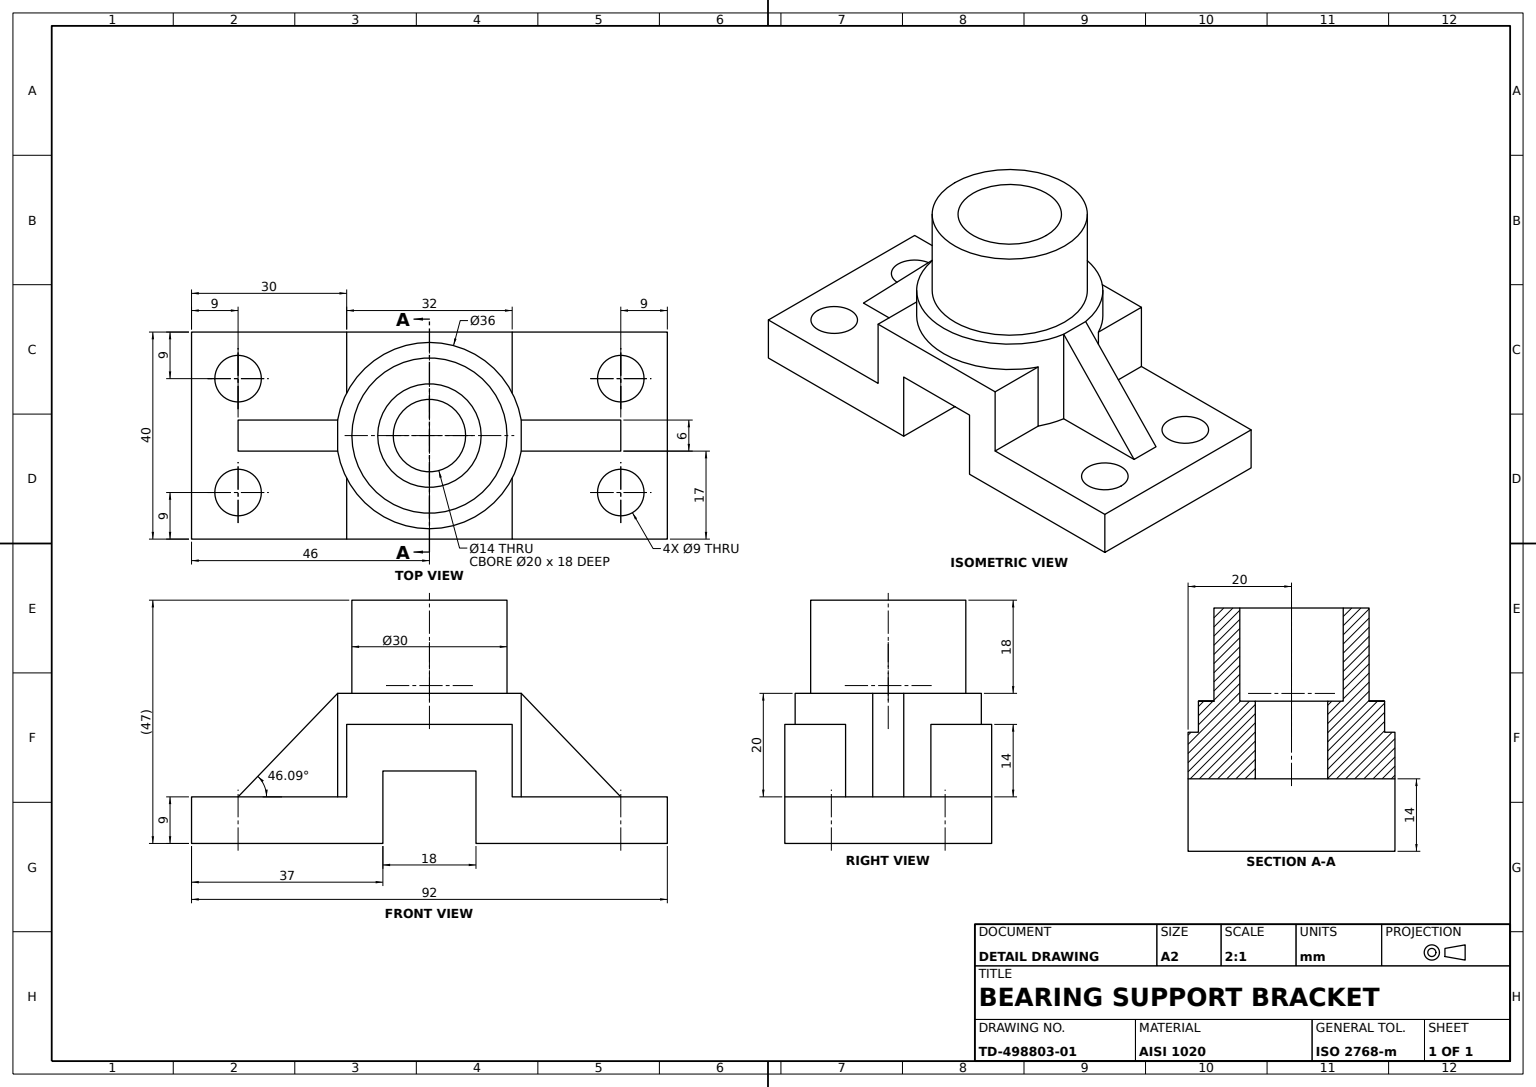
from build123d import *

# Parameters (mm, degrees)
STEPPED_BASE_DEPTH          = 20
COLLAR_36_SKETCH_R          = 18
COLLAR_36_DEPTH             = 20
COLLAR_TRIM_SKETCH_W        = 18
COLLAR_TRIM_SKETCH_H        = 5
COLLAR_TRIM_CUT_DEPTH       = 68.505555327
HUB_30_SKETCH_R             = 15
HUB_30_DEPTH                = 18
COUNTERBORE_20_SKETCH_R     = 10
COUNTERBORE_20_DEPTH        = 18
BORE_14_SKETCH_R            = 7
BORE_14_DEPTH               = 58.939623747
MOUNTING_HOLE_9_SKETCH_R    = 4.5
MOUNTING_HOLES_9_DEPTH      = 63.92853089
SUPPORT_START               = -20
SUPPORT_RIB_DEPTH           = 20
RIB_TRIM_CUT_DEPTH          = 70.670653793
MIRRORED_RIB_TRIM_CUT_DEPTH = 70.670653793


with BuildPart() as part:
    # Base Profile Sketch → Stepped Base (new, symmetric)
    with BuildSketch(Plane.XY):
        Polygon((-46, 0), (-9, 0), (-9, 14), (9, 14), (9, 0), (46, 0), (46, 9), (16, 9), (16, 23), (-16, 23), (-16, 9), (-46, 9), align=None)
    extrude(amount=STEPPED_BASE_DEPTH, both=True)

    # Collar Ø36 Sketch → Collar Ø36 (add)
    with BuildSketch(Plane(origin=(0, 9, 0), x_dir=(1, 0, 0), z_dir=(0, 1, 0))):
        with Locations(Location((0, 0, 0), (0, 0, 27.266044451))):
            Circle(COLLAR_36_SKETCH_R)
    extrude(amount=COLLAR_36_DEPTH)

    # Collar Trim Sketch → Collar Trim Cut (cut, through all)
    with BuildSketch(Plane.XY.offset(20)):
        with Locations((0, 11.5)):
            Rectangle(COLLAR_TRIM_SKETCH_W, COLLAR_TRIM_SKETCH_H)
    extrude(amount=-COLLAR_TRIM_CUT_DEPTH, mode=Mode.SUBTRACT)

    # Hub Ø30 Sketch → Hub Ø30 (add)
    with BuildSketch(Plane(origin=(0, 29, 0), x_dir=(1, 0, 0), z_dir=(0, 1, 0))):
        with Locations(Location((0, 0, 0), (0, 0, 180))):
            Circle(HUB_30_SKETCH_R)
    extrude(amount=HUB_30_DEPTH)

    # Counterbore Ø20 Sketch → Counterbore Ø20 (cut)
    with BuildSketch(Plane(origin=(0, 47, 0), x_dir=(1, 0, 0), z_dir=(0, 1, 0))):
        with Locations(Location((0, 0, 0), (0, 0, 180))):
            Circle(COUNTERBORE_20_SKETCH_R)
    extrude(amount=-COUNTERBORE_20_DEPTH, mode=Mode.SUBTRACT)

    # Bore Ø14 Sketch → Bore Ø14 (cut, through all)
    with BuildSketch(Plane(origin=(0, 29, 0), x_dir=(1, 0, 0), z_dir=(0, 1, 0))):
        with Locations(Location((0, 0, 0), (0, 0, 180))):
            Circle(BORE_14_SKETCH_R)
    extrude(amount=-BORE_14_DEPTH, mode=Mode.SUBTRACT)

    # Mounting Hole Ø9 Sketch → Mounting Holes Ø9 (cut, through all)
    with BuildSketch(Plane(origin=(0, 9, 0), x_dir=(1, 0, 0), z_dir=(0, 1, 0))):
        with Locations(Location((37, -11, 0), (0, 0, 180))):
            Circle(MOUNTING_HOLE_9_SKETCH_R)
        with Locations(Location((37, 11, 0), (0, 0, 180))):
            Circle(MOUNTING_HOLE_9_SKETCH_R)
    mounting_holes_9 = extrude(amount=-MOUNTING_HOLES_9_DEPTH, mode=Mode.SUBTRACT)

    # Support Rib Sketch → Support Rib (add)
    with BuildSketch(Plane(origin=(0, 29, 0), x_dir=(1, 0, 0), z_dir=(0, 1, 0)).offset(SUPPORT_START)):
        with BuildLine():
            Line((37, 3), (37, -3))
            Line((37, -3), (17.748239349, -3))
            ThreePointArc((17.748239349, -3), (18, 0), (17.748239349, 3))
            Line((17.748239349, 3), (37, 3))
        make_face()
    support_rib = extrude(amount=SUPPORT_RIB_DEPTH)

    # Rib Trim Sketch → Rib Trim Cut (cut, through all)
    with BuildSketch(Plane.XY.offset(3)):
        Polygon((17.748239349, 29), (37, 9), (37, 29), align=None)
    extrude(amount=-RIB_TRIM_CUT_DEPTH, mode=Mode.SUBTRACT)

    # Rib and Holes Mirror: Mounting Holes Ø9, Support Rib across plane
    add(mounting_holes_9.mirror(Plane(origin=(0, 0, 0), x_dir=(0, 0, 1), z_dir=(1, 0, 0))), mode=Mode.SUBTRACT)
    add(support_rib.mirror(Plane(origin=(0, 0, 0), x_dir=(0, 0, 1), z_dir=(1, 0, 0))))

    # Mirrored Rib Trim Sketch → Mirrored Rib Trim Cut (cut, through all)
    with BuildSketch(Plane.XY.offset(3)):
        Polygon((-17.748239349, 29), (-37, 9), (-37, 29), align=None)
    extrude(amount=-MIRRORED_RIB_TRIM_CUT_DEPTH, mode=Mode.SUBTRACT)


solid = part.part
